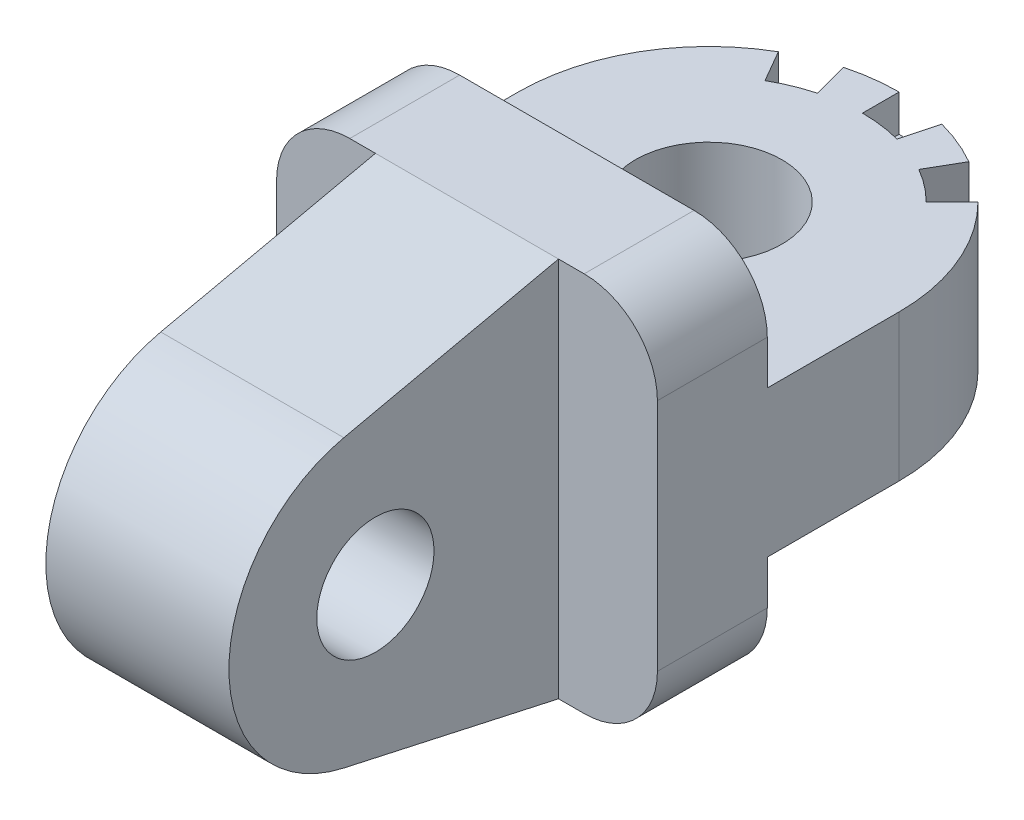
ISO-10303-21;
HEADER;
FILE_DESCRIPTION(('STEP AP214'),'2;1');
FILE_NAME('part.step','',(''),(''),'','','');
FILE_SCHEMA(('AUTOMOTIVE_DESIGN { 1 0 10303 214 1 1 1 1 }'));
ENDSEC;
DATA;
#1=APPLICATION_CONTEXT('core data for automotive mechanical design processes');
#2=APPLICATION_PROTOCOL_DEFINITION('international standard','automotive_design',2000,#1);
#3=PRODUCT_CONTEXT('',#1,'mechanical');
#4=PRODUCT('Part','Part','',(#3));
#5=PRODUCT_RELATED_PRODUCT_CATEGORY('part','',(#4));
#6=PRODUCT_DEFINITION_FORMATION('','',#4);
#7=PRODUCT_DEFINITION_CONTEXT('part definition',#1,'design');
#8=PRODUCT_DEFINITION('design','',#6,#7);
#9=PRODUCT_DEFINITION_SHAPE('','',#8);
#10=(LENGTH_UNIT() NAMED_UNIT(*) SI_UNIT(.MILLI.,.METRE.));
#11=(NAMED_UNIT(*) PLANE_ANGLE_UNIT() SI_UNIT($,.RADIAN.));
#12=(NAMED_UNIT(*) SI_UNIT($,.STERADIAN.) SOLID_ANGLE_UNIT());
#13=UNCERTAINTY_MEASURE_WITH_UNIT(LENGTH_MEASURE(1.E-05),#10,'distance_accuracy_value','');
#14=(GEOMETRIC_REPRESENTATION_CONTEXT(3) GLOBAL_UNCERTAINTY_ASSIGNED_CONTEXT((#13)) GLOBAL_UNIT_ASSIGNED_CONTEXT((#10,
#11,#12)) REPRESENTATION_CONTEXT('',''));
#15=CARTESIAN_POINT('',(0.,0.,0.));
#16=DIRECTION('',(0.,0.,1.));
#17=DIRECTION('',(1.,0.,0.));
#18=AXIS2_PLACEMENT_3D('',#15,#16,#17);
#19=CARTESIAN_POINT('',(0.,0.,-18.));
#20=DIRECTION('',(0.,1.,0.));
#21=DIRECTION('',(-1.,0.,0.));
#22=AXIS2_PLACEMENT_3D('',#19,#20,#21);
#23=CYLINDRICAL_SURFACE('',#22,26.);
#24=CARTESIAN_POINT('',(0.,36.,-18.));
#25=DIRECTION('',(0.,1.,0.));
#26=DIRECTION('',(-1.,0.,0.));
#27=AXIS2_PLACEMENT_3D('',#24,#25,#26);
#28=CIRCLE('',#27,26.);
#29=CARTESIAN_POINT('',(-13.,36.,-40.5166604983954));
#30=VERTEX_POINT('',#29);
#31=CARTESIAN_POINT('',(-26.,36.,-18.));
#32=VERTEX_POINT('',#31);
#33=EDGE_CURVE('E352',#30,#32,#28,.T.);
#34=ORIENTED_EDGE('',*,*,#33,.F.);
#35=DIRECTION('',(0.,1.,0.));
#36=VECTOR('',#35,1.);
#37=CARTESIAN_POINT('',(-13.,31.,-40.5166604983954));
#38=LINE('',#37,#36);
#39=CARTESIAN_POINT('',(-13.,31.,-40.5166604983954));
#40=VERTEX_POINT('',#39);
#41=EDGE_CURVE('E268',#40,#30,#38,.T.);
#42=ORIENTED_EDGE('',*,*,#41,.F.);
#43=CARTESIAN_POINT('',(0.,31.,-18.));
#44=DIRECTION('',(0.,1.,0.));
#45=DIRECTION('',(-1.,0.,0.));
#46=AXIS2_PLACEMENT_3D('',#43,#44,#45);
#47=CIRCLE('',#46,26.);
#48=CARTESIAN_POINT('',(-6.72929517266555,31.,-43.1140714835158));
#49=VERTEX_POINT('',#48);
#50=EDGE_CURVE('E251',#49,#40,#47,.T.);
#51=ORIENTED_EDGE('',*,*,#50,.F.);
#52=DIRECTION('',(0.,1.,0.));
#53=VECTOR('',#52,1.);
#54=CARTESIAN_POINT('',(-6.72929517266555,31.,-43.1140714835158));
#55=LINE('',#54,#53);
#56=CARTESIAN_POINT('',(-6.72929517266554,36.,-43.1140714835158));
#57=VERTEX_POINT('',#56);
#58=EDGE_CURVE('E238',#49,#57,#55,.T.);
#59=ORIENTED_EDGE('',*,*,#58,.T.);
#60=CARTESIAN_POINT('',(0.,36.,-44.));
#61=VERTEX_POINT('',#60);
#62=EDGE_CURVE('E552',#61,#57,#28,.T.);
#63=ORIENTED_EDGE('',*,*,#62,.F.);
#64=DIRECTION('',(0.,1.,0.));
#65=VECTOR('',#64,1.);
#66=CARTESIAN_POINT('',(0.,31.,-44.));
#67=LINE('',#66,#65);
#68=CARTESIAN_POINT('',(0.,31.,-44.));
#69=VERTEX_POINT('',#68);
#70=EDGE_CURVE('E292',#69,#61,#67,.T.);
#71=ORIENTED_EDGE('',*,*,#70,.F.);
#72=CARTESIAN_POINT('',(0.,31.,-18.));
#73=DIRECTION('',(0.,1.,0.));
#74=DIRECTION('',(-1.,0.,0.));
#75=AXIS2_PLACEMENT_3D('',#72,#73,#74);
#76=CIRCLE('',#75,26.);
#77=CARTESIAN_POINT('',(6.7292951726655,31.,-43.1140714835158));
#78=VERTEX_POINT('',#77);
#79=EDGE_CURVE('E279',#78,#69,#76,.T.);
#80=ORIENTED_EDGE('',*,*,#79,.F.);
#81=DIRECTION('',(0.,1.,0.));
#82=VECTOR('',#81,1.);
#83=CARTESIAN_POINT('',(6.7292951726655,31.,-43.1140714835158));
#84=LINE('',#83,#82);
#85=CARTESIAN_POINT('',(6.7292951726655,36.,-43.1140714835158));
#86=VERTEX_POINT('',#85);
#87=EDGE_CURVE('E291',#78,#86,#84,.T.);
#88=ORIENTED_EDGE('',*,*,#87,.T.);
#89=CARTESIAN_POINT('',(13.,36.,-40.5166604983954));
#90=VERTEX_POINT('',#89);
#91=EDGE_CURVE('E357',#90,#86,#28,.T.);
#92=ORIENTED_EDGE('',*,*,#91,.F.);
#93=DIRECTION('',(0.,1.,0.));
#94=VECTOR('',#93,1.);
#95=CARTESIAN_POINT('',(13.,31.,-40.5166604983954));
#96=LINE('',#95,#94);
#97=CARTESIAN_POINT('',(13.,31.,-40.5166604983954));
#98=VERTEX_POINT('',#97);
#99=EDGE_CURVE('E319',#98,#90,#96,.T.);
#100=ORIENTED_EDGE('',*,*,#99,.F.);
#101=CARTESIAN_POINT('',(0.,31.,-18.));
#102=DIRECTION('',(0.,1.,0.));
#103=DIRECTION('',(-1.,0.,0.));
#104=AXIS2_PLACEMENT_3D('',#101,#102,#103);
#105=CIRCLE('',#104,26.);
#106=CARTESIAN_POINT('',(18.3847763108502,31.,-36.3847763108502));
#107=VERTEX_POINT('',#106);
#108=EDGE_CURVE('E304',#107,#98,#105,.T.);
#109=ORIENTED_EDGE('',*,*,#108,.F.);
#110=DIRECTION('',(0.,1.,0.));
#111=VECTOR('',#110,1.);
#112=CARTESIAN_POINT('',(18.3847763108502,31.,-36.3847763108502));
#113=LINE('',#112,#111);
#114=CARTESIAN_POINT('',(18.3847763108502,36.,-36.3847763108502));
#115=VERTEX_POINT('',#114);
#116=EDGE_CURVE('E325',#107,#115,#113,.T.);
#117=ORIENTED_EDGE('',*,*,#116,.T.);
#118=CARTESIAN_POINT('',(26.,36.,-18.));
#119=VERTEX_POINT('',#118);
#120=EDGE_CURVE('E355',#119,#115,#28,.T.);
#121=ORIENTED_EDGE('',*,*,#120,.F.);
#122=DIRECTION('',(0.,1.,0.));
#123=VECTOR('',#122,1.);
#124=CARTESIAN_POINT('',(26.,0.,-18.));
#125=LINE('',#124,#123);
#126=CARTESIAN_POINT('',(26.,16.,-18.));
#127=VERTEX_POINT('',#126);
#128=EDGE_CURVE('E363',#127,#119,#125,.T.);
#129=ORIENTED_EDGE('',*,*,#128,.F.);
#130=CARTESIAN_POINT('',(0.,16.,-18.));
#131=DIRECTION('',(0.,-1.,0.));
#132=DIRECTION('',(0.,0.,-1.));
#133=AXIS2_PLACEMENT_3D('',#130,#131,#132);
#134=CIRCLE('',#133,26.);
#135=CARTESIAN_POINT('',(-26.,16.,-18.));
#136=VERTEX_POINT('',#135);
#137=EDGE_CURVE('E328',#136,#127,#134,.T.);
#138=ORIENTED_EDGE('',*,*,#137,.F.);
#139=DIRECTION('',(0.,1.,0.));
#140=VECTOR('',#139,1.);
#141=CARTESIAN_POINT('',(-26.,0.,-18.));
#142=LINE('',#141,#140);
#143=EDGE_CURVE('E361',#136,#32,#142,.T.);
#144=ORIENTED_EDGE('',*,*,#143,.T.);
#145=EDGE_LOOP('',(#34,#42,#51,#59,#63,#71,#80,#88,#92,#100,#109,#117,#121,#129,#138,#144));
#146=FACE_BOUND('',#145,.T.);
#147=ADVANCED_FACE('F44',(#146),#23,.T.);
#148=CARTESIAN_POINT('',(0.,36.,-18.));
#149=DIRECTION('',(0.,1.,0.));
#150=DIRECTION('',(-1.,0.,0.));
#151=AXIS2_PLACEMENT_3D('',#148,#149,#150);
#152=PLANE('',#151);
#153=CARTESIAN_POINT('',(0.,36.,-18.));
#154=DIRECTION('',(0.,1.,0.));
#155=DIRECTION('',(-1.,0.,0.));
#156=AXIS2_PLACEMENT_3D('',#153,#154,#155);
#157=CIRCLE('',#156,10.);
#158=CARTESIAN_POINT('',(-9.99999999999999,36.,-18.));
#159=VERTEX_POINT('',#158);
#160=EDGE_CURVE('E447',#159,#159,#157,.T.);
#161=ORIENTED_EDGE('',*,*,#160,.F.);
#162=EDGE_LOOP('',(#161));
#163=FACE_BOUND('',#162,.T.);
#164=CARTESIAN_POINT('',(0.,36.,-18.));
#165=DIRECTION('',(0.,1.,0.));
#166=DIRECTION('',(-1.,0.,0.));
#167=AXIS2_PLACEMENT_3D('',#164,#165,#166);
#168=CIRCLE('',#167,21.);
#169=CARTESIAN_POINT('',(-5.43519994715293,36.,-38.2844423520704));
#170=VERTEX_POINT('',#169);
#171=CARTESIAN_POINT('',(-10.5,36.,-36.1865334794732));
#172=VERTEX_POINT('',#171);
#173=EDGE_CURVE('E65',#170,#172,#168,.T.);
#174=ORIENTED_EDGE('',*,*,#173,.T.);
#175=DIRECTION('',(-0.500000000000002,0.,-0.866025403784438));
#176=VECTOR('',#175,1.);
#177=CARTESIAN_POINT('',(7.79422863405998,36.,-4.50000000000003));
#178=LINE('',#177,#176);
#179=EDGE_CURVE('E249',#172,#30,#178,.T.);
#180=ORIENTED_EDGE('',*,*,#179,.T.);
#181=ORIENTED_EDGE('',*,*,#33,.T.);
#182=DIRECTION('',(0.,0.,1.));
#183=VECTOR('',#182,1.);
#184=CARTESIAN_POINT('',(-26.,36.,0.));
#185=LINE('',#184,#183);
#186=CARTESIAN_POINT('',(-26.,36.,0.));
#187=VERTEX_POINT('',#186);
#188=EDGE_CURVE('E345',#32,#187,#185,.T.);
#189=ORIENTED_EDGE('',*,*,#188,.T.);
#190=DIRECTION('',(1.,0.,0.));
#191=VECTOR('',#190,1.);
#192=CARTESIAN_POINT('',(-26.,36.,0.));
#193=LINE('',#192,#191);
#194=CARTESIAN_POINT('',(26.,36.,0.));
#195=VERTEX_POINT('',#194);
#196=EDGE_CURVE('E341',#187,#195,#193,.T.);
#197=ORIENTED_EDGE('',*,*,#196,.T.);
#198=DIRECTION('',(0.,0.,-1.));
#199=VECTOR('',#198,1.);
#200=CARTESIAN_POINT('',(26.,36.,0.));
#201=LINE('',#200,#199);
#202=EDGE_CURVE('E346',#195,#119,#201,.T.);
#203=ORIENTED_EDGE('',*,*,#202,.T.);
#204=ORIENTED_EDGE('',*,*,#120,.T.);
#205=DIRECTION('',(0.707106781186549,0.,-0.707106781186547));
#206=VECTOR('',#205,1.);
#207=CARTESIAN_POINT('',(-9.00000000000002,36.,-9.00000000000006));
#208=LINE('',#207,#206);
#209=CARTESIAN_POINT('',(14.8492424049176,36.,-32.8492424049175));
#210=VERTEX_POINT('',#209);
#211=EDGE_CURVE('E311',#210,#115,#208,.T.);
#212=ORIENTED_EDGE('',*,*,#211,.F.);
#213=CARTESIAN_POINT('',(0.,36.,-18.));
#214=DIRECTION('',(0.,1.,0.));
#215=DIRECTION('',(-1.,0.,0.));
#216=AXIS2_PLACEMENT_3D('',#213,#214,#215);
#217=CIRCLE('',#216,21.);
#218=CARTESIAN_POINT('',(10.5,36.,-36.1865334794732));
#219=VERTEX_POINT('',#218);
#220=EDGE_CURVE('E309',#210,#219,#217,.T.);
#221=ORIENTED_EDGE('',*,*,#220,.T.);
#222=DIRECTION('',(0.500000000000001,0.,-0.866025403784438));
#223=VECTOR('',#222,1.);
#224=CARTESIAN_POINT('',(-7.79422863406001,36.,-4.50000000000005));
#225=LINE('',#224,#223);
#226=EDGE_CURVE('E302',#219,#90,#225,.T.);
#227=ORIENTED_EDGE('',*,*,#226,.T.);
#228=ORIENTED_EDGE('',*,*,#91,.T.);
#229=DIRECTION('',(0.258819045102521,0.,-0.965925826289068));
#230=VECTOR('',#229,1.);
#231=CARTESIAN_POINT('',(-4.50000000000006,36.,-1.20577136594008));
#232=LINE('',#231,#230);
#233=CARTESIAN_POINT('',(5.43519994715297,36.,-38.2844423520704));
#234=VERTEX_POINT('',#233);
#235=EDGE_CURVE('E281',#234,#86,#232,.T.);
#236=ORIENTED_EDGE('',*,*,#235,.F.);
#237=CARTESIAN_POINT('',(0.,36.,-18.));
#238=DIRECTION('',(0.,1.,0.));
#239=DIRECTION('',(-1.,0.,0.));
#240=AXIS2_PLACEMENT_3D('',#237,#238,#239);
#241=CIRCLE('',#240,21.);
#242=CARTESIAN_POINT('',(0.,36.,-39.));
#243=VERTEX_POINT('',#242);
#244=EDGE_CURVE('E66',#234,#243,#241,.T.);
#245=ORIENTED_EDGE('',*,*,#244,.T.);
#246=DIRECTION('',(0.,0.,-1.));
#247=VECTOR('',#246,1.);
#248=CARTESIAN_POINT('',(0.,36.,0.));
#249=LINE('',#248,#247);
#250=EDGE_CURVE('E274',#243,#61,#249,.T.);
#251=ORIENTED_EDGE('',*,*,#250,.T.);
#252=ORIENTED_EDGE('',*,*,#62,.T.);
#253=DIRECTION('',(-0.258819045102521,0.,-0.965925826289068));
#254=VECTOR('',#253,1.);
#255=CARTESIAN_POINT('',(4.50000000000001,36.,-1.20577136594005));
#256=LINE('',#255,#254);
#257=EDGE_CURVE('E257',#170,#57,#256,.T.);
#258=ORIENTED_EDGE('',*,*,#257,.F.);
#259=EDGE_LOOP('',(#174,#180,#181,#189,#197,#203,#204,#212,#221,#227,#228,#236,#245,#251,#252,#258));
#260=FACE_BOUND('',#259,.T.);
#261=ADVANCED_FACE('F530',(#163,#260),#152,.T.);
#262=CARTESIAN_POINT('',(26.,52.,15.));
#263=DIRECTION('',(0.,0.976492352797987,0.215552046909908));
#264=DIRECTION('',(0.,-0.215552046909908,0.976492352797987));
#265=AXIS2_PLACEMENT_3D('',#262,#263,#264);
#266=PLANE('',#265);
#267=DIRECTION('',(-1.,0.,0.));
#268=VECTOR('',#267,1.);
#269=CARTESIAN_POINT('',(26.,45.5298470559597,44.3110409381982));
#270=LINE('',#269,#268);
#271=CARTESIAN_POINT('',(12.5,45.5298470559597,44.3110409381982));
#272=VERTEX_POINT('',#271);
#273=CARTESIAN_POINT('',(-12.5,45.5298470559597,44.3110409381982));
#274=VERTEX_POINT('',#273);
#275=EDGE_CURVE('E397',#272,#274,#270,.T.);
#276=ORIENTED_EDGE('',*,*,#275,.F.);
#277=DIRECTION('',(0.,-0.215552046909908,0.976492352797987));
#278=VECTOR('',#277,1.);
#279=CARTESIAN_POINT('',(12.5,52.,15.));
#280=LINE('',#279,#278);
#281=CARTESIAN_POINT('',(12.5,52.,15.));
#282=VERTEX_POINT('',#281);
#283=EDGE_CURVE('E366',#282,#272,#280,.T.);
#284=ORIENTED_EDGE('',*,*,#283,.F.);
#285=DIRECTION('',(-1.,0.,0.));
#286=VECTOR('',#285,1.);
#287=CARTESIAN_POINT('',(15.9999999999999,52.,15.));
#288=LINE('',#287,#286);
#289=CARTESIAN_POINT('',(-12.5,52.,15.));
#290=VERTEX_POINT('',#289);
#291=EDGE_CURVE('E412',#282,#290,#288,.T.);
#292=ORIENTED_EDGE('',*,*,#291,.T.);
#293=DIRECTION('',(0.,0.215552046909908,-0.976492352797987));
#294=VECTOR('',#293,1.);
#295=CARTESIAN_POINT('',(-12.5,52.,15.));
#296=LINE('',#295,#294);
#297=EDGE_CURVE('E386',#274,#290,#296,.T.);
#298=ORIENTED_EDGE('',*,*,#297,.F.);
#299=EDGE_LOOP('',(#276,#284,#292,#298));
#300=FACE_BOUND('',#299,.T.);
#301=ADVANCED_FACE('F486',(#300),#266,.T.);
#302=CARTESIAN_POINT('',(26.,26.,40.));
#303=DIRECTION('',(-1.,0.,0.));
#304=DIRECTION('',(0.,-1.,0.));
#305=AXIS2_PLACEMENT_3D('',#302,#303,#304);
#306=CYLINDRICAL_SURFACE('',#305,20.);
#307=DIRECTION('',(-1.,0.,0.));
#308=VECTOR('',#307,1.);
#309=CARTESIAN_POINT('',(26.,6.47015294404022,44.3110409381981));
#310=LINE('',#309,#308);
#311=CARTESIAN_POINT('',(12.5,6.47015294404022,44.3110409381981));
#312=VERTEX_POINT('',#311);
#313=CARTESIAN_POINT('',(-12.5,6.47015294404023,44.3110409381981));
#314=VERTEX_POINT('',#313);
#315=EDGE_CURVE('E391',#312,#314,#310,.T.);
#316=ORIENTED_EDGE('',*,*,#315,.F.);
#317=CARTESIAN_POINT('',(12.5,26.,40.));
#318=DIRECTION('',(1.,0.,0.));
#319=DIRECTION('',(0.,1.,0.));
#320=AXIS2_PLACEMENT_3D('',#317,#318,#319);
#321=CIRCLE('',#320,20.);
#322=EDGE_CURVE('E367',#272,#312,#321,.T.);
#323=ORIENTED_EDGE('',*,*,#322,.F.);
#324=ORIENTED_EDGE('',*,*,#275,.T.);
#325=CARTESIAN_POINT('',(-12.5,26.,40.));
#326=DIRECTION('',(-1.,0.,0.));
#327=DIRECTION('',(0.,-1.,0.));
#328=AXIS2_PLACEMENT_3D('',#325,#326,#327);
#329=CIRCLE('',#328,20.);
#330=EDGE_CURVE('E387',#314,#274,#329,.T.);
#331=ORIENTED_EDGE('',*,*,#330,.F.);
#332=EDGE_LOOP('',(#316,#323,#324,#331));
#333=FACE_BOUND('',#332,.T.);
#334=ADVANCED_FACE('F483',(#333),#306,.T.);
#335=CARTESIAN_POINT('',(26.,0.,15.));
#336=DIRECTION('',(0.,-0.976492352797988,0.215552046909906));
#337=DIRECTION('',(0.,-0.215552046909906,-0.976492352797988));
#338=AXIS2_PLACEMENT_3D('',#335,#336,#337);
#339=PLANE('',#338);
#340=DIRECTION('',(1.,0.,0.));
#341=VECTOR('',#340,1.);
#342=CARTESIAN_POINT('',(-16.,0.,15.));
#343=LINE('',#342,#341);
#344=CARTESIAN_POINT('',(-12.5,0.,15.));
#345=VERTEX_POINT('',#344);
#346=CARTESIAN_POINT('',(12.5,0.,15.));
#347=VERTEX_POINT('',#346);
#348=EDGE_CURVE('E405',#345,#347,#343,.T.);
#349=ORIENTED_EDGE('',*,*,#348,.T.);
#350=DIRECTION('',(0.,-0.215552046909906,-0.976492352797988));
#351=VECTOR('',#350,1.);
#352=CARTESIAN_POINT('',(12.5,0.,15.));
#353=LINE('',#352,#351);
#354=EDGE_CURVE('E375',#312,#347,#353,.T.);
#355=ORIENTED_EDGE('',*,*,#354,.F.);
#356=ORIENTED_EDGE('',*,*,#315,.T.);
#357=DIRECTION('',(0.,0.215552046909906,0.976492352797988));
#358=VECTOR('',#357,1.);
#359=CARTESIAN_POINT('',(-12.5,0.,15.));
#360=LINE('',#359,#358);
#361=EDGE_CURVE('E382',#345,#314,#360,.T.);
#362=ORIENTED_EDGE('',*,*,#361,.F.);
#363=EDGE_LOOP('',(#349,#355,#356,#362));
#364=FACE_BOUND('',#363,.T.);
#365=ADVANCED_FACE('F508',(#364),#339,.T.);
#366=CARTESIAN_POINT('',(-16.,10.,15.));
#367=DIRECTION('',(0.,0.,-1.));
#368=DIRECTION('',(-1.,0.,0.));
#369=AXIS2_PLACEMENT_3D('',#366,#367,#368);
#370=CYLINDRICAL_SURFACE('',#369,10.);
#371=CARTESIAN_POINT('',(-16.,10.,0.));
#372=DIRECTION('',(0.,0.,1.));
#373=DIRECTION('',(-1.,0.,0.));
#374=AXIS2_PLACEMENT_3D('',#371,#372,#373);
#375=CIRCLE('',#374,10.);
#376=CARTESIAN_POINT('',(-26.,10.,0.));
#377=VERTEX_POINT('',#376);
#378=CARTESIAN_POINT('',(-16.,0.,0.));
#379=VERTEX_POINT('',#378);
#380=EDGE_CURVE('E398',#377,#379,#375,.T.);
#381=ORIENTED_EDGE('',*,*,#380,.T.);
#382=DIRECTION('',(0.,0.,-1.));
#383=VECTOR('',#382,1.);
#384=CARTESIAN_POINT('',(-16.,0.,15.));
#385=LINE('',#384,#383);
#386=CARTESIAN_POINT('',(-16.,0.,15.));
#387=VERTEX_POINT('',#386);
#388=EDGE_CURVE('E11',#387,#379,#385,.T.);
#389=ORIENTED_EDGE('',*,*,#388,.F.);
#390=CARTESIAN_POINT('',(-16.,10.,15.));
#391=DIRECTION('',(0.,0.,1.));
#392=DIRECTION('',(-1.,0.,0.));
#393=AXIS2_PLACEMENT_3D('',#390,#391,#392);
#394=CIRCLE('',#393,10.);
#395=CARTESIAN_POINT('',(-26.,10.,15.));
#396=VERTEX_POINT('',#395);
#397=EDGE_CURVE('E396',#396,#387,#394,.T.);
#398=ORIENTED_EDGE('',*,*,#397,.F.);
#399=DIRECTION('',(0.,0.,-1.));
#400=VECTOR('',#399,1.);
#401=CARTESIAN_POINT('',(-26.,10.,15.));
#402=LINE('',#401,#400);
#403=EDGE_CURVE('E418',#396,#377,#402,.T.);
#404=ORIENTED_EDGE('',*,*,#403,.T.);
#405=EDGE_LOOP('',(#381,#389,#398,#404));
#406=FACE_BOUND('',#405,.T.);
#407=ADVANCED_FACE('F50',(#406),#370,.T.);
#408=CARTESIAN_POINT('',(-16.,0.,15.));
#409=DIRECTION('',(0.,1.,0.));
#410=DIRECTION('',(0.,0.,1.));
#411=AXIS2_PLACEMENT_3D('',#408,#409,#410);
#412=PLANE('',#411);
#413=ORIENTED_EDGE('',*,*,#388,.T.);
#414=DIRECTION('',(-1.,0.,0.));
#415=VECTOR('',#414,1.);
#416=CARTESIAN_POINT('',(-26.,0.,0.));
#417=LINE('',#416,#415);
#418=CARTESIAN_POINT('',(16.,0.,0.));
#419=VERTEX_POINT('',#418);
#420=EDGE_CURVE('E270',#419,#379,#417,.T.);
#421=ORIENTED_EDGE('',*,*,#420,.F.);
#422=DIRECTION('',(0.,0.,-1.));
#423=VECTOR('',#422,1.);
#424=CARTESIAN_POINT('',(16.,0.,15.));
#425=LINE('',#424,#423);
#426=CARTESIAN_POINT('',(16.,0.,15.));
#427=VERTEX_POINT('',#426);
#428=EDGE_CURVE('E53',#427,#419,#425,.T.);
#429=ORIENTED_EDGE('',*,*,#428,.F.);
#430=DIRECTION('',(1.,0.,0.));
#431=VECTOR('',#430,1.);
#432=CARTESIAN_POINT('',(12.5,0.,15.));
#433=LINE('',#432,#431);
#434=EDGE_CURVE('E380',#347,#427,#433,.T.);
#435=ORIENTED_EDGE('',*,*,#434,.F.);
#436=ORIENTED_EDGE('',*,*,#348,.F.);
#437=EDGE_CURVE('E404',#387,#345,#343,.T.);
#438=ORIENTED_EDGE('',*,*,#437,.F.);
#439=EDGE_LOOP('',(#413,#421,#429,#435,#436,#438));
#440=FACE_BOUND('',#439,.T.);
#441=ADVANCED_FACE('F506',(#440),#412,.F.);
#442=CARTESIAN_POINT('',(16.,10.,15.));
#443=DIRECTION('',(0.,0.,-1.));
#444=DIRECTION('',(-1.,0.,0.));
#445=AXIS2_PLACEMENT_3D('',#442,#443,#444);
#446=CYLINDRICAL_SURFACE('',#445,10.);
#447=CARTESIAN_POINT('',(16.,10.,0.));
#448=DIRECTION('',(0.,0.,1.));
#449=DIRECTION('',(1.,0.,0.));
#450=AXIS2_PLACEMENT_3D('',#447,#448,#449);
#451=CIRCLE('',#450,10.);
#452=CARTESIAN_POINT('',(26.,10.,0.));
#453=VERTEX_POINT('',#452);
#454=EDGE_CURVE('E420',#419,#453,#451,.T.);
#455=ORIENTED_EDGE('',*,*,#454,.T.);
#456=DIRECTION('',(0.,0.,-1.));
#457=VECTOR('',#456,1.);
#458=CARTESIAN_POINT('',(26.,10.,15.));
#459=LINE('',#458,#457);
#460=CARTESIAN_POINT('',(26.,9.99999999999999,15.));
#461=VERTEX_POINT('',#460);
#462=EDGE_CURVE('E442',#461,#453,#459,.T.);
#463=ORIENTED_EDGE('',*,*,#462,.F.);
#464=CARTESIAN_POINT('',(16.,10.,15.));
#465=DIRECTION('',(0.,0.,1.));
#466=DIRECTION('',(1.,0.,0.));
#467=AXIS2_PLACEMENT_3D('',#464,#465,#466);
#468=CIRCLE('',#467,10.);
#469=EDGE_CURVE('E410',#427,#461,#468,.T.);
#470=ORIENTED_EDGE('',*,*,#469,.F.);
#471=ORIENTED_EDGE('',*,*,#428,.T.);
#472=EDGE_LOOP('',(#455,#463,#470,#471));
#473=FACE_BOUND('',#472,.T.);
#474=ADVANCED_FACE('F899',(#473),#446,.T.);
#475=CARTESIAN_POINT('',(26.,10.,15.));
#476=DIRECTION('',(-1.,0.,0.));
#477=DIRECTION('',(0.,-1.,0.));
#478=AXIS2_PLACEMENT_3D('',#475,#476,#477);
#479=PLANE('',#478);
#480=ORIENTED_EDGE('',*,*,#462,.T.);
#481=DIRECTION('',(0.,-1.,0.));
#482=VECTOR('',#481,1.);
#483=CARTESIAN_POINT('',(26.,16.,0.));
#484=LINE('',#483,#482);
#485=CARTESIAN_POINT('',(26.,16.,0.));
#486=VERTEX_POINT('',#485);
#487=EDGE_CURVE('E333',#486,#453,#484,.T.);
#488=ORIENTED_EDGE('',*,*,#487,.F.);
#489=DIRECTION('',(0.,0.,1.));
#490=VECTOR('',#489,1.);
#491=CARTESIAN_POINT('',(26.,16.,0.));
#492=LINE('',#491,#490);
#493=EDGE_CURVE('E332',#127,#486,#492,.T.);
#494=ORIENTED_EDGE('',*,*,#493,.F.);
#495=ORIENTED_EDGE('',*,*,#128,.T.);
#496=ORIENTED_EDGE('',*,*,#202,.F.);
#497=DIRECTION('',(0.,1.,0.));
#498=VECTOR('',#497,1.);
#499=CARTESIAN_POINT('',(26.,36.,0.));
#500=LINE('',#499,#498);
#501=CARTESIAN_POINT('',(26.,42.,0.));
#502=VERTEX_POINT('',#501);
#503=EDGE_CURVE('E358',#195,#502,#500,.T.);
#504=ORIENTED_EDGE('',*,*,#503,.T.);
#505=DIRECTION('',(0.,0.,-1.));
#506=VECTOR('',#505,1.);
#507=CARTESIAN_POINT('',(26.,41.9999999999999,15.));
#508=LINE('',#507,#506);
#509=CARTESIAN_POINT('',(26.,42.,15.));
#510=VERTEX_POINT('',#509);
#511=EDGE_CURVE('E437',#510,#502,#508,.T.);
#512=ORIENTED_EDGE('',*,*,#511,.F.);
#513=DIRECTION('',(0.,1.,0.));
#514=VECTOR('',#513,1.);
#515=CARTESIAN_POINT('',(26.,52.,15.));
#516=LINE('',#515,#514);
#517=EDGE_CURVE('E368',#461,#510,#516,.T.);
#518=ORIENTED_EDGE('',*,*,#517,.F.);
#519=EDGE_LOOP('',(#480,#488,#494,#495,#496,#504,#512,#518));
#520=FACE_BOUND('',#519,.T.);
#521=ADVANCED_FACE('F524',(#520),#479,.F.);
#522=CARTESIAN_POINT('',(16.,42.,15.));
#523=DIRECTION('',(0.,0.,-1.));
#524=DIRECTION('',(-1.,0.,0.));
#525=AXIS2_PLACEMENT_3D('',#522,#523,#524);
#526=CYLINDRICAL_SURFACE('',#525,10.);
#527=CARTESIAN_POINT('',(16.,42.,0.));
#528=DIRECTION('',(0.,0.,1.));
#529=DIRECTION('',(1.,0.,0.));
#530=AXIS2_PLACEMENT_3D('',#527,#528,#529);
#531=CIRCLE('',#530,10.);
#532=CARTESIAN_POINT('',(16.,52.,0.));
#533=VERTEX_POINT('',#532);
#534=EDGE_CURVE('E425',#502,#533,#531,.T.);
#535=ORIENTED_EDGE('',*,*,#534,.T.);
#536=DIRECTION('',(0.,0.,-1.));
#537=VECTOR('',#536,1.);
#538=CARTESIAN_POINT('',(15.9999999999999,52.,15.));
#539=LINE('',#538,#537);
#540=CARTESIAN_POINT('',(15.9999999999999,52.,15.));
#541=VERTEX_POINT('',#540);
#542=EDGE_CURVE('E434',#541,#533,#539,.T.);
#543=ORIENTED_EDGE('',*,*,#542,.F.);
#544=CARTESIAN_POINT('',(16.,42.,15.));
#545=DIRECTION('',(0.,0.,1.));
#546=DIRECTION('',(1.,0.,0.));
#547=AXIS2_PLACEMENT_3D('',#544,#545,#546);
#548=CIRCLE('',#547,10.);
#549=EDGE_CURVE('E409',#510,#541,#548,.T.);
#550=ORIENTED_EDGE('',*,*,#549,.F.);
#551=ORIENTED_EDGE('',*,*,#511,.T.);
#552=EDGE_LOOP('',(#535,#543,#550,#551));
#553=FACE_BOUND('',#552,.T.);
#554=ADVANCED_FACE('F519',(#553),#526,.T.);
#555=CARTESIAN_POINT('',(15.9999999999999,52.,15.));
#556=DIRECTION('',(0.,-1.,0.));
#557=DIRECTION('',(1.,0.,0.));
#558=AXIS2_PLACEMENT_3D('',#555,#556,#557);
#559=PLANE('',#558);
#560=ORIENTED_EDGE('',*,*,#542,.T.);
#561=DIRECTION('',(1.,0.,0.));
#562=VECTOR('',#561,1.);
#563=CARTESIAN_POINT('',(-26.,52.,0.));
#564=LINE('',#563,#562);
#565=CARTESIAN_POINT('',(-16.,52.,0.));
#566=VERTEX_POINT('',#565);
#567=EDGE_CURVE('E336',#566,#533,#564,.T.);
#568=ORIENTED_EDGE('',*,*,#567,.F.);
#569=DIRECTION('',(0.,0.,-1.));
#570=VECTOR('',#569,1.);
#571=CARTESIAN_POINT('',(-15.9999999999999,52.,15.));
#572=LINE('',#571,#570);
#573=CARTESIAN_POINT('',(-16.,52.,15.));
#574=VERTEX_POINT('',#573);
#575=EDGE_CURVE('E435',#574,#566,#572,.T.);
#576=ORIENTED_EDGE('',*,*,#575,.F.);
#577=DIRECTION('',(-1.,0.,0.));
#578=VECTOR('',#577,1.);
#579=CARTESIAN_POINT('',(-12.5,52.,15.));
#580=LINE('',#579,#578);
#581=EDGE_CURVE('E395',#290,#574,#580,.T.);
#582=ORIENTED_EDGE('',*,*,#581,.F.);
#583=ORIENTED_EDGE('',*,*,#291,.F.);
#584=EDGE_CURVE('E415',#541,#282,#288,.T.);
#585=ORIENTED_EDGE('',*,*,#584,.F.);
#586=EDGE_LOOP('',(#560,#568,#576,#582,#583,#585));
#587=FACE_BOUND('',#586,.T.);
#588=ADVANCED_FACE('F492',(#587),#559,.F.);
#589=CARTESIAN_POINT('',(-16.,42.,15.));
#590=DIRECTION('',(0.,0.,-1.));
#591=DIRECTION('',(-1.,0.,0.));
#592=AXIS2_PLACEMENT_3D('',#589,#590,#591);
#593=CYLINDRICAL_SURFACE('',#592,10.);
#594=CARTESIAN_POINT('',(-16.,42.,0.));
#595=DIRECTION('',(0.,0.,1.));
#596=DIRECTION('',(1.,0.,0.));
#597=AXIS2_PLACEMENT_3D('',#594,#595,#596);
#598=CIRCLE('',#597,10.);
#599=CARTESIAN_POINT('',(-26.,42.,0.));
#600=VERTEX_POINT('',#599);
#601=EDGE_CURVE('E401',#566,#600,#598,.T.);
#602=ORIENTED_EDGE('',*,*,#601,.T.);
#603=DIRECTION('',(0.,0.,-1.));
#604=VECTOR('',#603,1.);
#605=CARTESIAN_POINT('',(-26.,42.,15.));
#606=LINE('',#605,#604);
#607=CARTESIAN_POINT('',(-26.,42.,15.));
#608=VERTEX_POINT('',#607);
#609=EDGE_CURVE('E427',#608,#600,#606,.T.);
#610=ORIENTED_EDGE('',*,*,#609,.F.);
#611=CARTESIAN_POINT('',(-16.,42.,15.));
#612=DIRECTION('',(0.,0.,1.));
#613=DIRECTION('',(1.,0.,0.));
#614=AXIS2_PLACEMENT_3D('',#611,#612,#613);
#615=CIRCLE('',#614,10.);
#616=EDGE_CURVE('E414',#574,#608,#615,.T.);
#617=ORIENTED_EDGE('',*,*,#616,.F.);
#618=ORIENTED_EDGE('',*,*,#575,.T.);
#619=EDGE_LOOP('',(#602,#610,#617,#618));
#620=FACE_BOUND('',#619,.T.);
#621=ADVANCED_FACE('F563',(#620),#593,.T.);
#622=CARTESIAN_POINT('',(-26.,41.9999999999999,15.));
#623=DIRECTION('',(1.,0.,0.));
#624=DIRECTION('',(0.,1.,0.));
#625=AXIS2_PLACEMENT_3D('',#622,#623,#624);
#626=PLANE('',#625);
#627=DIRECTION('',(0.,0.,-1.));
#628=VECTOR('',#627,1.);
#629=CARTESIAN_POINT('',(-26.,16.,0.));
#630=LINE('',#629,#628);
#631=CARTESIAN_POINT('',(-26.,16.,0.));
#632=VERTEX_POINT('',#631);
#633=EDGE_CURVE('E330',#632,#136,#630,.T.);
#634=ORIENTED_EDGE('',*,*,#633,.F.);
#635=DIRECTION('',(0.,-1.,0.));
#636=VECTOR('',#635,1.);
#637=CARTESIAN_POINT('',(-26.,16.,0.));
#638=LINE('',#637,#636);
#639=EDGE_CURVE('E340',#632,#377,#638,.T.);
#640=ORIENTED_EDGE('',*,*,#639,.T.);
#641=ORIENTED_EDGE('',*,*,#403,.F.);
#642=DIRECTION('',(0.,-1.,0.));
#643=VECTOR('',#642,1.);
#644=CARTESIAN_POINT('',(-26.,52.,15.));
#645=LINE('',#644,#643);
#646=EDGE_CURVE('E379',#608,#396,#645,.T.);
#647=ORIENTED_EDGE('',*,*,#646,.F.);
#648=ORIENTED_EDGE('',*,*,#609,.T.);
#649=DIRECTION('',(0.,1.,0.));
#650=VECTOR('',#649,1.);
#651=CARTESIAN_POINT('',(-26.,36.,0.));
#652=LINE('',#651,#650);
#653=EDGE_CURVE('E351',#187,#600,#652,.T.);
#654=ORIENTED_EDGE('',*,*,#653,.F.);
#655=ORIENTED_EDGE('',*,*,#188,.F.);
#656=ORIENTED_EDGE('',*,*,#143,.F.);
#657=EDGE_LOOP('',(#634,#640,#641,#647,#648,#654,#655,#656));
#658=FACE_BOUND('',#657,.T.);
#659=ADVANCED_FACE('F556',(#658),#626,.F.);
#660=CARTESIAN_POINT('',(-12.5,52.,15.));
#661=DIRECTION('',(0.,0.,-1.));
#662=DIRECTION('',(-1.,0.,0.));
#663=AXIS2_PLACEMENT_3D('',#660,#661,#662);
#664=PLANE('',#663);
#665=ORIENTED_EDGE('',*,*,#437,.T.);
#666=DIRECTION('',(0.,-1.,0.));
#667=VECTOR('',#666,1.);
#668=CARTESIAN_POINT('',(-12.5,52.,15.));
#669=LINE('',#668,#667);
#670=EDGE_CURVE('E381',#290,#345,#669,.T.);
#671=ORIENTED_EDGE('',*,*,#670,.F.);
#672=ORIENTED_EDGE('',*,*,#581,.T.);
#673=ORIENTED_EDGE('',*,*,#616,.T.);
#674=ORIENTED_EDGE('',*,*,#646,.T.);
#675=ORIENTED_EDGE('',*,*,#397,.T.);
#676=EDGE_LOOP('',(#665,#671,#672,#673,#674,#675));
#677=FACE_BOUND('',#676,.T.);
#678=ADVANCED_FACE('F499',(#677),#664,.F.);
#679=CARTESIAN_POINT('',(-12.5,26.,40.));
#680=DIRECTION('',(-1.,0.,0.));
#681=DIRECTION('',(0.,-1.,0.));
#682=AXIS2_PLACEMENT_3D('',#679,#680,#681);
#683=PLANE('',#682);
#684=CARTESIAN_POINT('',(-12.5,26.,40.));
#685=DIRECTION('',(-1.,0.,0.));
#686=DIRECTION('',(0.,-1.,0.));
#687=AXIS2_PLACEMENT_3D('',#684,#685,#686);
#688=CIRCLE('',#687,12.5);
#689=CARTESIAN_POINT('',(-12.5,13.5,40.));
#690=VERTEX_POINT('',#689);
#691=EDGE_CURVE('E454',#690,#690,#688,.T.);
#692=ORIENTED_EDGE('',*,*,#691,.F.);
#693=EDGE_LOOP('',(#692));
#694=FACE_BOUND('',#693,.T.);
#695=ORIENTED_EDGE('',*,*,#670,.T.);
#696=ORIENTED_EDGE('',*,*,#361,.T.);
#697=ORIENTED_EDGE('',*,*,#330,.T.);
#698=ORIENTED_EDGE('',*,*,#297,.T.);
#699=EDGE_LOOP('',(#695,#696,#697,#698));
#700=FACE_BOUND('',#699,.T.);
#701=ADVANCED_FACE('F489',(#694,#700),#683,.T.);
#702=CARTESIAN_POINT('',(12.5,52.,15.));
#703=DIRECTION('',(0.,0.,-1.));
#704=DIRECTION('',(-1.,0.,0.));
#705=AXIS2_PLACEMENT_3D('',#702,#703,#704);
#706=PLANE('',#705);
#707=ORIENTED_EDGE('',*,*,#517,.T.);
#708=ORIENTED_EDGE('',*,*,#549,.T.);
#709=ORIENTED_EDGE('',*,*,#584,.T.);
#710=DIRECTION('',(0.,1.,0.));
#711=VECTOR('',#710,1.);
#712=CARTESIAN_POINT('',(12.5,52.,15.));
#713=LINE('',#712,#711);
#714=EDGE_CURVE('E372',#347,#282,#713,.T.);
#715=ORIENTED_EDGE('',*,*,#714,.F.);
#716=ORIENTED_EDGE('',*,*,#434,.T.);
#717=ORIENTED_EDGE('',*,*,#469,.T.);
#718=EDGE_LOOP('',(#707,#708,#709,#715,#716,#717));
#719=FACE_BOUND('',#718,.T.);
#720=ADVANCED_FACE('F472',(#719),#706,.F.);
#721=CARTESIAN_POINT('',(12.5,26.,40.));
#722=DIRECTION('',(1.,0.,0.));
#723=DIRECTION('',(0.,1.,0.));
#724=AXIS2_PLACEMENT_3D('',#721,#722,#723);
#725=PLANE('',#724);
#726=CARTESIAN_POINT('',(12.5,26.,40.));
#727=DIRECTION('',(1.,0.,0.));
#728=DIRECTION('',(0.,1.,0.));
#729=AXIS2_PLACEMENT_3D('',#726,#727,#728);
#730=CIRCLE('',#729,8.);
#731=CARTESIAN_POINT('',(12.5,34.,40.));
#732=VERTEX_POINT('',#731);
#733=EDGE_CURVE('E47',#732,#732,#730,.T.);
#734=ORIENTED_EDGE('',*,*,#733,.F.);
#735=EDGE_LOOP('',(#734));
#736=FACE_BOUND('',#735,.T.);
#737=ORIENTED_EDGE('',*,*,#283,.T.);
#738=ORIENTED_EDGE('',*,*,#322,.T.);
#739=ORIENTED_EDGE('',*,*,#354,.T.);
#740=ORIENTED_EDGE('',*,*,#714,.T.);
#741=EDGE_LOOP('',(#737,#738,#739,#740));
#742=FACE_BOUND('',#741,.T.);
#743=ADVANCED_FACE('F468',(#736,#742),#725,.T.);
#744=CARTESIAN_POINT('',(-26.,36.,0.));
#745=DIRECTION('',(0.,0.,1.));
#746=DIRECTION('',(1.,0.,0.));
#747=AXIS2_PLACEMENT_3D('',#744,#745,#746);
#748=PLANE('',#747);
#749=ORIENTED_EDGE('',*,*,#503,.F.);
#750=ORIENTED_EDGE('',*,*,#196,.F.);
#751=ORIENTED_EDGE('',*,*,#653,.T.);
#752=ORIENTED_EDGE('',*,*,#601,.F.);
#753=ORIENTED_EDGE('',*,*,#567,.T.);
#754=ORIENTED_EDGE('',*,*,#534,.F.);
#755=EDGE_LOOP('',(#749,#750,#751,#752,#753,#754));
#756=FACE_BOUND('',#755,.T.);
#757=ADVANCED_FACE('F473',(#756),#748,.F.);
#758=CARTESIAN_POINT('',(-26.,16.,0.));
#759=DIRECTION('',(0.,0.,1.));
#760=DIRECTION('',(1.,0.,0.));
#761=AXIS2_PLACEMENT_3D('',#758,#759,#760);
#762=PLANE('',#761);
#763=ORIENTED_EDGE('',*,*,#639,.F.);
#764=DIRECTION('',(-1.,0.,0.));
#765=VECTOR('',#764,1.);
#766=CARTESIAN_POINT('',(-26.,16.,0.));
#767=LINE('',#766,#765);
#768=EDGE_CURVE('E334',#486,#632,#767,.T.);
#769=ORIENTED_EDGE('',*,*,#768,.F.);
#770=ORIENTED_EDGE('',*,*,#487,.T.);
#771=ORIENTED_EDGE('',*,*,#454,.F.);
#772=ORIENTED_EDGE('',*,*,#420,.T.);
#773=ORIENTED_EDGE('',*,*,#380,.F.);
#774=EDGE_LOOP('',(#763,#769,#770,#771,#772,#773));
#775=FACE_BOUND('',#774,.T.);
#776=ADVANCED_FACE('F654',(#775),#762,.F.);
#777=CARTESIAN_POINT('',(0.,16.,-18.));
#778=DIRECTION('',(0.,-1.,0.));
#779=DIRECTION('',(0.,0.,-1.));
#780=AXIS2_PLACEMENT_3D('',#777,#778,#779);
#781=PLANE('',#780);
#782=CARTESIAN_POINT('',(0.,16.,-18.));
#783=DIRECTION('',(0.,-1.,0.));
#784=DIRECTION('',(0.,0.,-1.));
#785=AXIS2_PLACEMENT_3D('',#782,#783,#784);
#786=CIRCLE('',#785,10.);
#787=CARTESIAN_POINT('',(0.,16.,-28.));
#788=VERTEX_POINT('',#787);
#789=EDGE_CURVE('E314',#788,#788,#786,.T.);
#790=ORIENTED_EDGE('',*,*,#789,.F.);
#791=EDGE_LOOP('',(#790));
#792=FACE_BOUND('',#791,.T.);
#793=ORIENTED_EDGE('',*,*,#633,.T.);
#794=ORIENTED_EDGE('',*,*,#137,.T.);
#795=ORIENTED_EDGE('',*,*,#493,.T.);
#796=ORIENTED_EDGE('',*,*,#768,.T.);
#797=EDGE_LOOP('',(#793,#794,#795,#796));
#798=FACE_BOUND('',#797,.T.);
#799=ADVANCED_FACE('F661',(#792,#798),#781,.T.);
#800=CARTESIAN_POINT('',(0.,31.,-18.));
#801=DIRECTION('',(0.,1.,0.));
#802=DIRECTION('',(-1.,0.,0.));
#803=AXIS2_PLACEMENT_3D('',#800,#801,#802);
#804=CYLINDRICAL_SURFACE('',#803,21.);
#805=ORIENTED_EDGE('',*,*,#220,.F.);
#806=DIRECTION('',(0.,1.,0.));
#807=VECTOR('',#806,1.);
#808=CARTESIAN_POINT('',(14.8492424049175,31.,-32.8492424049175));
#809=LINE('',#808,#807);
#810=CARTESIAN_POINT('',(14.8492424049175,31.,-32.8492424049175));
#811=VERTEX_POINT('',#810);
#812=EDGE_CURVE('E310',#811,#210,#809,.T.);
#813=ORIENTED_EDGE('',*,*,#812,.F.);
#814=CARTESIAN_POINT('',(0.,31.,-18.));
#815=DIRECTION('',(0.,1.,0.));
#816=DIRECTION('',(-1.,0.,0.));
#817=AXIS2_PLACEMENT_3D('',#814,#815,#816);
#818=CIRCLE('',#817,21.);
#819=CARTESIAN_POINT('',(10.5,31.,-36.1865334794732));
#820=VERTEX_POINT('',#819);
#821=EDGE_CURVE('E300',#811,#820,#818,.T.);
#822=ORIENTED_EDGE('',*,*,#821,.T.);
#823=DIRECTION('',(0.,1.,0.));
#824=VECTOR('',#823,1.);
#825=CARTESIAN_POINT('',(10.5,31.,-36.1865334794732));
#826=LINE('',#825,#824);
#827=EDGE_CURVE('E287',#820,#219,#826,.T.);
#828=ORIENTED_EDGE('',*,*,#827,.T.);
#829=EDGE_LOOP('',(#805,#813,#822,#828));
#830=FACE_BOUND('',#829,.T.);
#831=ADVANCED_FACE('F542',(#830),#804,.T.);
#832=CARTESIAN_POINT('',(-7.79422863406001,31.,-4.50000000000005));
#833=DIRECTION('',(0.866025403784438,0.,0.500000000000001));
#834=DIRECTION('',(0.500000000000001,0.,-0.866025403784438));
#835=AXIS2_PLACEMENT_3D('',#832,#833,#834);
#836=PLANE('',#835);
#837=ORIENTED_EDGE('',*,*,#226,.F.);
#838=ORIENTED_EDGE('',*,*,#827,.F.);
#839=DIRECTION('',(0.500000000000001,0.,-0.866025403784438));
#840=VECTOR('',#839,1.);
#841=CARTESIAN_POINT('',(-7.79422863406001,31.,-4.50000000000005));
#842=LINE('',#841,#840);
#843=EDGE_CURVE('E307',#820,#98,#842,.T.);
#844=ORIENTED_EDGE('',*,*,#843,.T.);
#845=ORIENTED_EDGE('',*,*,#99,.T.);
#846=EDGE_LOOP('',(#837,#838,#844,#845));
#847=FACE_BOUND('',#846,.T.);
#848=ADVANCED_FACE('F546',(#847),#836,.T.);
#849=CARTESIAN_POINT('',(-9.00000000000002,31.,-9.00000000000006));
#850=DIRECTION('',(0.707106781186547,0.,0.707106781186549));
#851=DIRECTION('',(0.707106781186549,0.,-0.707106781186547));
#852=AXIS2_PLACEMENT_3D('',#849,#850,#851);
#853=PLANE('',#852);
#854=ORIENTED_EDGE('',*,*,#211,.T.);
#855=ORIENTED_EDGE('',*,*,#116,.F.);
#856=DIRECTION('',(0.707106781186549,0.,-0.707106781186547));
#857=VECTOR('',#856,1.);
#858=CARTESIAN_POINT('',(-9.00000000000002,31.,-9.00000000000006));
#859=LINE('',#858,#857);
#860=EDGE_CURVE('E296',#811,#107,#859,.T.);
#861=ORIENTED_EDGE('',*,*,#860,.F.);
#862=ORIENTED_EDGE('',*,*,#812,.T.);
#863=EDGE_LOOP('',(#854,#855,#861,#862));
#864=FACE_BOUND('',#863,.T.);
#865=ADVANCED_FACE('F538',(#864),#853,.F.);
#866=CARTESIAN_POINT('',(0.,31.,0.));
#867=DIRECTION('',(0.,1.,0.));
#868=DIRECTION('',(-1.,0.,0.));
#869=AXIS2_PLACEMENT_3D('',#866,#867,#868);
#870=PLANE('',#869);
#871=ORIENTED_EDGE('',*,*,#821,.F.);
#872=ORIENTED_EDGE('',*,*,#860,.T.);
#873=ORIENTED_EDGE('',*,*,#108,.T.);
#874=ORIENTED_EDGE('',*,*,#843,.F.);
#875=EDGE_LOOP('',(#871,#872,#873,#874));
#876=FACE_BOUND('',#875,.T.);
#877=ADVANCED_FACE('F541',(#876),#870,.T.);
#878=CARTESIAN_POINT('',(0.,31.,-18.));
#879=DIRECTION('',(0.,1.,0.));
#880=DIRECTION('',(-1.,0.,0.));
#881=AXIS2_PLACEMENT_3D('',#878,#879,#880);
#882=CYLINDRICAL_SURFACE('',#881,21.);
#883=ORIENTED_EDGE('',*,*,#244,.F.);
#884=DIRECTION('',(0.,1.,0.));
#885=VECTOR('',#884,1.);
#886=CARTESIAN_POINT('',(5.43519994715289,31.,-38.2844423520704));
#887=LINE('',#886,#885);
#888=CARTESIAN_POINT('',(5.43519994715289,31.,-38.2844423520704));
#889=VERTEX_POINT('',#888);
#890=EDGE_CURVE('E283',#889,#234,#887,.T.);
#891=ORIENTED_EDGE('',*,*,#890,.F.);
#892=CARTESIAN_POINT('',(0.,31.,-18.));
#893=DIRECTION('',(0.,1.,0.));
#894=DIRECTION('',(-1.,0.,0.));
#895=AXIS2_PLACEMENT_3D('',#892,#893,#894);
#896=CIRCLE('',#895,21.);
#897=CARTESIAN_POINT('',(0.,31.,-39.));
#898=VERTEX_POINT('',#897);
#899=EDGE_CURVE('E271',#889,#898,#896,.T.);
#900=ORIENTED_EDGE('',*,*,#899,.T.);
#901=DIRECTION('',(0.,1.,0.));
#902=VECTOR('',#901,1.);
#903=CARTESIAN_POINT('',(0.,31.,-39.));
#904=LINE('',#903,#902);
#905=EDGE_CURVE('E261',#898,#243,#904,.T.);
#906=ORIENTED_EDGE('',*,*,#905,.T.);
#907=EDGE_LOOP('',(#883,#891,#900,#906));
#908=FACE_BOUND('',#907,.T.);
#909=ADVANCED_FACE('F723',(#908),#882,.T.);
#910=CARTESIAN_POINT('',(0.,31.,0.));
#911=DIRECTION('',(1.,0.,0.));
#912=DIRECTION('',(0.,1.,0.));
#913=AXIS2_PLACEMENT_3D('',#910,#911,#912);
#914=PLANE('',#913);
#915=ORIENTED_EDGE('',*,*,#250,.F.);
#916=ORIENTED_EDGE('',*,*,#905,.F.);
#917=DIRECTION('',(0.,0.,-1.));
#918=VECTOR('',#917,1.);
#919=CARTESIAN_POINT('',(0.,31.,0.));
#920=LINE('',#919,#918);
#921=EDGE_CURVE('E282',#898,#69,#920,.T.);
#922=ORIENTED_EDGE('',*,*,#921,.T.);
#923=ORIENTED_EDGE('',*,*,#70,.T.);
#924=EDGE_LOOP('',(#915,#916,#922,#923));
#925=FACE_BOUND('',#924,.T.);
#926=ADVANCED_FACE('F734',(#925),#914,.T.);
#927=CARTESIAN_POINT('',(-4.50000000000007,31.,-1.20577136594008));
#928=DIRECTION('',(0.965925826289068,0.,0.258819045102521));
#929=DIRECTION('',(0.258819045102521,0.,-0.965925826289068));
#930=AXIS2_PLACEMENT_3D('',#927,#928,#929);
#931=PLANE('',#930);
#932=ORIENTED_EDGE('',*,*,#235,.T.);
#933=ORIENTED_EDGE('',*,*,#87,.F.);
#934=DIRECTION('',(0.258819045102521,0.,-0.965925826289068));
#935=VECTOR('',#934,1.);
#936=CARTESIAN_POINT('',(-4.50000000000007,31.,-1.20577136594008));
#937=LINE('',#936,#935);
#938=EDGE_CURVE('E273',#889,#78,#937,.T.);
#939=ORIENTED_EDGE('',*,*,#938,.F.);
#940=ORIENTED_EDGE('',*,*,#890,.T.);
#941=EDGE_LOOP('',(#932,#933,#939,#940));
#942=FACE_BOUND('',#941,.T.);
#943=ADVANCED_FACE('F741',(#942),#931,.F.);
#944=CARTESIAN_POINT('',(0.,31.,0.));
#945=DIRECTION('',(0.,1.,0.));
#946=DIRECTION('',(-1.,0.,0.));
#947=AXIS2_PLACEMENT_3D('',#944,#945,#946);
#948=PLANE('',#947);
#949=ORIENTED_EDGE('',*,*,#899,.F.);
#950=ORIENTED_EDGE('',*,*,#938,.T.);
#951=ORIENTED_EDGE('',*,*,#79,.T.);
#952=ORIENTED_EDGE('',*,*,#921,.F.);
#953=EDGE_LOOP('',(#949,#950,#951,#952));
#954=FACE_BOUND('',#953,.T.);
#955=ADVANCED_FACE('F760',(#954),#948,.T.);
#956=CARTESIAN_POINT('',(0.,31.,-18.));
#957=DIRECTION('',(0.,1.,0.));
#958=DIRECTION('',(-1.,0.,0.));
#959=AXIS2_PLACEMENT_3D('',#956,#957,#958);
#960=CYLINDRICAL_SURFACE('',#959,21.);
#961=ORIENTED_EDGE('',*,*,#173,.F.);
#962=DIRECTION('',(0.,1.,0.));
#963=VECTOR('',#962,1.);
#964=CARTESIAN_POINT('',(-5.43519994715294,31.,-38.2844423520704));
#965=LINE('',#964,#963);
#966=CARTESIAN_POINT('',(-5.43519994715294,31.,-38.2844423520704));
#967=VERTEX_POINT('',#966);
#968=EDGE_CURVE('E235',#967,#170,#965,.T.);
#969=ORIENTED_EDGE('',*,*,#968,.F.);
#970=CARTESIAN_POINT('',(0.,31.,-18.));
#971=DIRECTION('',(0.,1.,0.));
#972=DIRECTION('',(-1.,0.,0.));
#973=AXIS2_PLACEMENT_3D('',#970,#971,#972);
#974=CIRCLE('',#973,21.);
#975=CARTESIAN_POINT('',(-10.5,31.,-36.1865334794732));
#976=VERTEX_POINT('',#975);
#977=EDGE_CURVE('E231',#967,#976,#974,.T.);
#978=ORIENTED_EDGE('',*,*,#977,.T.);
#979=DIRECTION('',(0.,1.,0.));
#980=VECTOR('',#979,1.);
#981=CARTESIAN_POINT('',(-10.5,31.,-36.1865334794732));
#982=LINE('',#981,#980);
#983=EDGE_CURVE('E264',#976,#172,#982,.T.);
#984=ORIENTED_EDGE('',*,*,#983,.T.);
#985=EDGE_LOOP('',(#961,#969,#978,#984));
#986=FACE_BOUND('',#985,.T.);
#987=ADVANCED_FACE('F234',(#986),#960,.T.);
#988=CARTESIAN_POINT('',(7.79422863405998,31.,-4.50000000000003));
#989=DIRECTION('',(0.866025403784438,0.,-0.500000000000002));
#990=DIRECTION('',(-0.500000000000002,0.,-0.866025403784438));
#991=AXIS2_PLACEMENT_3D('',#988,#989,#990);
#992=PLANE('',#991);
#993=ORIENTED_EDGE('',*,*,#179,.F.);
#994=ORIENTED_EDGE('',*,*,#983,.F.);
#995=DIRECTION('',(-0.500000000000002,0.,-0.866025403784438));
#996=VECTOR('',#995,1.);
#997=CARTESIAN_POINT('',(7.79422863405998,31.,-4.50000000000003));
#998=LINE('',#997,#996);
#999=EDGE_CURVE('E242',#976,#40,#998,.T.);
#1000=ORIENTED_EDGE('',*,*,#999,.T.);
#1001=ORIENTED_EDGE('',*,*,#41,.T.);
#1002=EDGE_LOOP('',(#993,#994,#1000,#1001));
#1003=FACE_BOUND('',#1002,.T.);
#1004=ADVANCED_FACE('F776',(#1003),#992,.T.);
#1005=CARTESIAN_POINT('',(4.5,31.,-1.20577136594005));
#1006=DIRECTION('',(0.965925826289068,0.,-0.258819045102521));
#1007=DIRECTION('',(-0.258819045102521,0.,-0.965925826289068));
#1008=AXIS2_PLACEMENT_3D('',#1005,#1006,#1007);
#1009=PLANE('',#1008);
#1010=ORIENTED_EDGE('',*,*,#257,.T.);
#1011=ORIENTED_EDGE('',*,*,#58,.F.);
#1012=DIRECTION('',(-0.258819045102521,0.,-0.965925826289068));
#1013=VECTOR('',#1012,1.);
#1014=CARTESIAN_POINT('',(4.5,31.,-1.20577136594005));
#1015=LINE('',#1014,#1013);
#1016=EDGE_CURVE('E250',#967,#49,#1015,.T.);
#1017=ORIENTED_EDGE('',*,*,#1016,.F.);
#1018=ORIENTED_EDGE('',*,*,#968,.T.);
#1019=EDGE_LOOP('',(#1010,#1011,#1017,#1018));
#1020=FACE_BOUND('',#1019,.T.);
#1021=ADVANCED_FACE('F253',(#1020),#1009,.F.);
#1022=CARTESIAN_POINT('',(0.,31.,0.));
#1023=DIRECTION('',(0.,1.,0.));
#1024=DIRECTION('',(-1.,0.,0.));
#1025=AXIS2_PLACEMENT_3D('',#1022,#1023,#1024);
#1026=PLANE('',#1025);
#1027=ORIENTED_EDGE('',*,*,#977,.F.);
#1028=ORIENTED_EDGE('',*,*,#1016,.T.);
#1029=ORIENTED_EDGE('',*,*,#50,.T.);
#1030=ORIENTED_EDGE('',*,*,#999,.F.);
#1031=EDGE_LOOP('',(#1027,#1028,#1029,#1030));
#1032=FACE_BOUND('',#1031,.T.);
#1033=ADVANCED_FACE('F241',(#1032),#1026,.T.);
#1034=CARTESIAN_POINT('',(0.,-14.,-18.));
#1035=DIRECTION('',(0.,1.,0.));
#1036=DIRECTION('',(-1.,0.,0.));
#1037=AXIS2_PLACEMENT_3D('',#1034,#1035,#1036);
#1038=CYLINDRICAL_SURFACE('',#1037,10.);
#1039=ORIENTED_EDGE('',*,*,#789,.T.);
#1040=EDGE_LOOP('',(#1039));
#1041=FACE_BOUND('',#1040,.T.);
#1042=ORIENTED_EDGE('',*,*,#160,.T.);
#1043=EDGE_LOOP('',(#1042));
#1044=FACE_BOUND('',#1043,.T.);
#1045=ADVANCED_FACE('F815',(#1041,#1044),#1038,.F.);
#1046=CARTESIAN_POINT('',(-9.5,26.,40.));
#1047=DIRECTION('',(-1.,0.,0.));
#1048=DIRECTION('',(0.,-1.,0.));
#1049=AXIS2_PLACEMENT_3D('',#1046,#1047,#1048);
#1050=CYLINDRICAL_SURFACE('',#1049,12.5);
#1051=CARTESIAN_POINT('',(-9.5,26.,40.));
#1052=DIRECTION('',(-1.,0.,0.));
#1053=DIRECTION('',(0.,-1.,0.));
#1054=AXIS2_PLACEMENT_3D('',#1051,#1052,#1053);
#1055=CIRCLE('',#1054,12.5);
#1056=CARTESIAN_POINT('',(-9.5,13.5,40.));
#1057=VERTEX_POINT('',#1056);
#1058=EDGE_CURVE('E446',#1057,#1057,#1055,.T.);
#1059=ORIENTED_EDGE('',*,*,#1058,.F.);
#1060=EDGE_LOOP('',(#1059));
#1061=FACE_BOUND('',#1060,.T.);
#1062=ORIENTED_EDGE('',*,*,#691,.T.);
#1063=EDGE_LOOP('',(#1062));
#1064=FACE_BOUND('',#1063,.T.);
#1065=ADVANCED_FACE('F825',(#1061,#1064),#1050,.F.);
#1066=CARTESIAN_POINT('',(-9.5,26.,40.));
#1067=DIRECTION('',(-1.,0.,0.));
#1068=DIRECTION('',(0.,-1.,0.));
#1069=AXIS2_PLACEMENT_3D('',#1066,#1067,#1068);
#1070=PLANE('',#1069);
#1071=CARTESIAN_POINT('',(-9.5,26.,40.));
#1072=DIRECTION('',(-1.,0.,0.));
#1073=DIRECTION('',(0.,-1.,0.));
#1074=AXIS2_PLACEMENT_3D('',#1071,#1072,#1073);
#1075=CIRCLE('',#1074,8.);
#1076=CARTESIAN_POINT('',(-9.5,18.,40.));
#1077=VERTEX_POINT('',#1076);
#1078=EDGE_CURVE('E459',#1077,#1077,#1075,.T.);
#1079=ORIENTED_EDGE('',*,*,#1078,.F.);
#1080=EDGE_LOOP('',(#1079));
#1081=FACE_BOUND('',#1080,.T.);
#1082=ORIENTED_EDGE('',*,*,#1058,.T.);
#1083=EDGE_LOOP('',(#1082));
#1084=FACE_BOUND('',#1083,.T.);
#1085=ADVANCED_FACE('F833',(#1081,#1084),#1070,.T.);
#1086=CARTESIAN_POINT('',(40.5,26.,40.));
#1087=DIRECTION('',(-1.,0.,0.));
#1088=DIRECTION('',(0.,-1.,0.));
#1089=AXIS2_PLACEMENT_3D('',#1086,#1087,#1088);
#1090=CYLINDRICAL_SURFACE('',#1089,8.);
#1091=ORIENTED_EDGE('',*,*,#733,.T.);
#1092=EDGE_LOOP('',(#1091));
#1093=FACE_BOUND('',#1092,.T.);
#1094=ORIENTED_EDGE('',*,*,#1078,.T.);
#1095=EDGE_LOOP('',(#1094));
#1096=FACE_BOUND('',#1095,.T.);
#1097=ADVANCED_FACE('F467',(#1093,#1096),#1090,.F.);
#1098=CLOSED_SHELL('',(#147,#261,#301,#334,#365,#407,#441,#474,#521,#554,#588,#621,#659,#678,
#701,#720,#743,#757,#776,#799,#831,#848,#865,#877,#909,#926,#943,#955,#987,#1004,#1021,#1033,
#1045,#1065,#1085,#1097));
#1099=MANIFOLD_SOLID_BREP('B2',#1098);
#1100=ADVANCED_BREP_SHAPE_REPRESENTATION('',(#18,#1099),#14);
#1101=SHAPE_DEFINITION_REPRESENTATION(#9,#1100);
ENDSEC;
END-ISO-10303-21;
